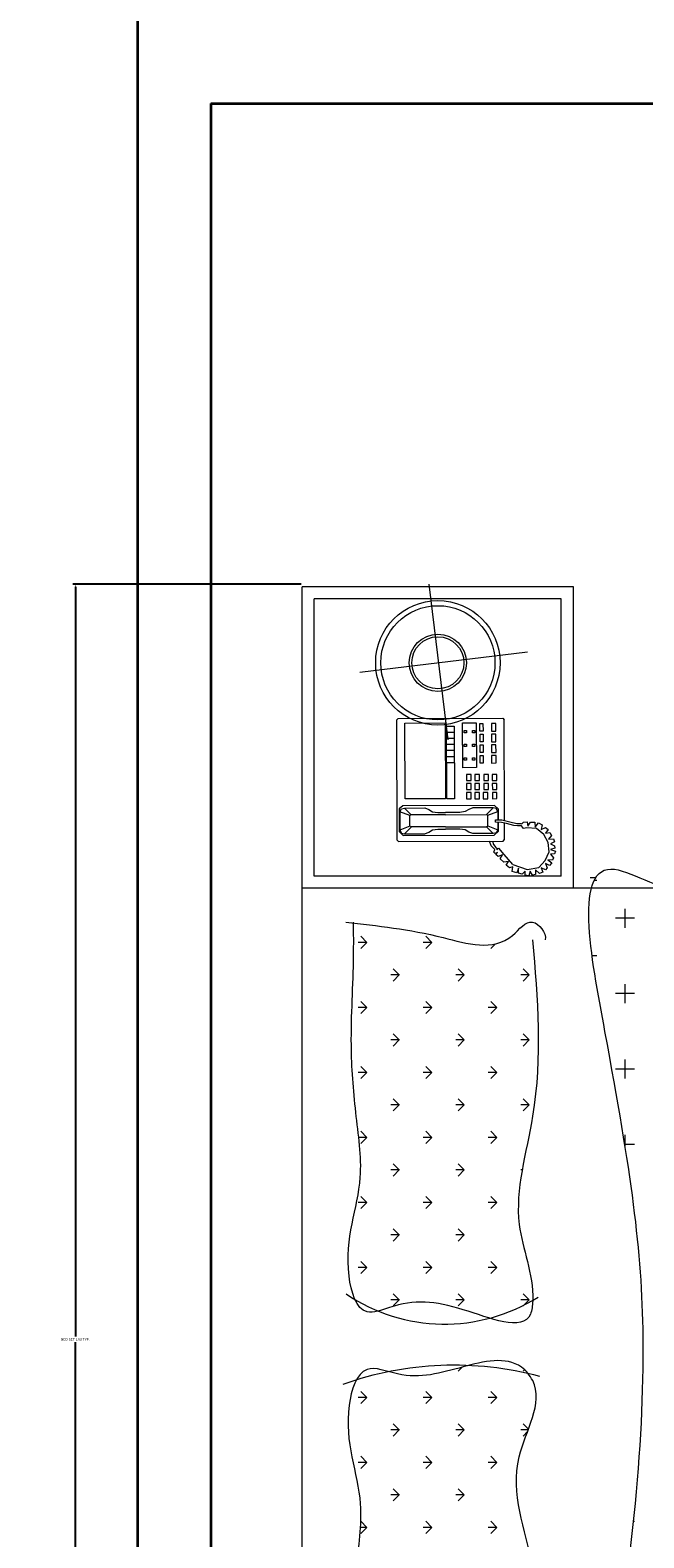
# Model space of a CAD drawing. Units: inches. Extents: x 3731 to 4318, y 1310 to 2388.
# Tile 4 of 57: x 3828 to 3870, y 1452 to 1554. Entities that reach past the tile are written whole.
import ezdxf

# ---------------------------------------------------------------- set-up
doc = ezdxf.new("R2010")
doc.units = ezdxf.units.IN
for name, color, linetype, lineweight in [('A-ANNO-DIMS', 2, 'Continuous', 18), ('A-FURN', 8, 'Continuous', 13), ('A-WALL', 7, 'Continuous', 35)]:
    doc.layers.add(name, color=color, linetype=linetype, lineweight=lineweight)
doc.styles.get("Standard").update_dxf_attribs({"font": 'arial.ttf'})
doc.dimstyles.get("Standard").update_dxf_attribs({"dimtxt": 0.18, "dimasz": 0.18, "dimexe": 0.18, "dimexo": 0.0625, "dimgap": 0.09, "dimtad": 0, "dimtih": 1, "dimtoh": 1, "dimdec": 4, "dimzin": 0, "dimdsep": 46, "dimtxsty": 'Standard', "dimcen": 0.09, "dimadec": 0, "dimazin": 0, "dimtfac": 1, "dimtdec": 4, "dimtofl": 0, "dimtmove": 0, "dimatfit": 3, "dimfxl": 1, "dimtolj": 1, "dimtzin": 0, "dimarcsym": 0})

# ---------------------------------------------------------------- blocks, each defined once
blk = doc.blocks.new('A$C200C7901')
for p, q in [((0.5, 2.3334), (2, 2.3334)), ((2, 2.3334), (2.5, 2.3334)), ((2, 1.6055), (2, 2.3334)), ((2.5, 1.8834), (2.5, 2.3334)), ((0.9943, 2.1721), (0.9842, 2.1822)), ((0.9943, 2.1721), (0.9842, 2.1822)), ((1.3176, 2.1721), (1.3075, 2.1822)), ((1.3176, 2.1721), (1.3075, 2.1822)), ((0.9943, 2.0643), (0.9842, 2.0744)), ((0.9943, 2.0643), (0.9842, 2.0744)), ((1.206, 2.0681), (1.1997, 2.0744)), ((1.206, 2.0681), (1.1997, 2.0744)), ((1.2019, 1.9645), (1.1997, 1.9666)), ((1.2019, 1.9645), (1.1997, 1.9666)), ((2, 1.8834), (2.5, 1.8834)), ((2.0171, 1.8467), (2.0171, 1.8556)), ((2.0171, 1.8467), (2.0171, 1.8556)), ((2.0129, 1.8445), (2.0129, 1.849)), ((2.0129, 1.8445), (2.0129, 1.849))]:
    blk.add_line(p, q)
at = {"linetype": 'ByBlock'}
for p, q in [((2.02, 2.3134), (2.48, 2.3134)), ((2.02, 1.9034), (2.02, 2.3134)), ((2.48, 1.9034), (2.48, 2.3134)), ((0.9404, 2.2259), (0.9303, 2.236)), ((0.9404, 2.2259), (0.9303, 2.236)), ((0.9404, 2.2259), (0.9404, 2.2369)), ((0.9404, 2.2259), (0.9404, 2.2369)), ((0.9404, 2.2259), (0.9505, 2.236)), ((0.9404, 2.2259), (0.9505, 2.236)), ((1.0482, 2.2259), (1.0381, 2.236)), ((1.0482, 2.2259), (1.0381, 2.236)), ((1.0482, 2.2259), (1.0482, 2.2402)), ((1.0482, 2.2259), (1.0482, 2.2402)), ((1.0482, 2.2259), (1.0583, 2.236)), ((1.0482, 2.2259), (1.0583, 2.236)), ((1.1559, 2.2259), (1.1458, 2.236)), ((1.1559, 2.2259), (1.1458, 2.236)), ((1.1559, 2.2259), (1.1559, 2.2402)), ((1.1559, 2.2259), (1.1559, 2.2402)), ((1.1559, 2.2259), (1.166, 2.236)), ((1.1559, 2.2259), (1.166, 2.236)), ((1.3714, 2.2259), (1.3613, 2.236)), ((1.3714, 2.2259), (1.3613, 2.236)), ((1.3714, 2.2259), (1.3714, 2.2402)), ((1.3714, 2.2259), (1.3714, 2.2402)), ((1.3714, 2.2259), (1.3815, 2.236)), ((1.3714, 2.2259), (1.3815, 2.236)), ((1.4792, 2.2259), (1.4691, 2.236)), ((1.4792, 2.2259), (1.4691, 2.236)), ((1.4792, 2.2259), (1.4792, 2.2402)), ((1.4792, 2.2259), (1.4792, 2.2402)), ((1.4792, 2.2259), (1.4893, 2.236)), ((1.4792, 2.2259), (1.4893, 2.236)), ((1.587, 2.2259), (1.5769, 2.236)), ((1.587, 2.2259), (1.5769, 2.236)), ((1.587, 2.2259), (1.587, 2.2393)), ((1.587, 2.2259), (1.587, 2.2393)), ((1.587, 2.2259), (1.5971, 2.236)), ((1.587, 2.2259), (1.5971, 2.236)), ((1.6947, 2.2259), (1.6846, 2.236)), ((1.6947, 2.2259), (1.6846, 2.236)), ((1.6947, 2.2259), (1.6947, 2.2402)), ((1.6947, 2.2259), (1.6947, 2.2402)), ((1.6947, 2.2259), (1.7048, 2.236)), ((1.6947, 2.2259), (1.7048, 2.236)), ((1.8025, 2.2259), (1.7924, 2.236)), ((1.8025, 2.2259), (1.7924, 2.236)), ((1.8025, 2.2259), (1.8025, 2.2402)), ((1.8025, 2.2259), (1.8025, 2.2402)), ((1.8025, 2.2259), (1.8126, 2.236)), ((1.8025, 2.2259), (1.8126, 2.236)), ((1.9103, 2.2259), (1.9002, 2.236)), ((1.9103, 2.2259), (1.9002, 2.236)), ((1.9103, 2.2259), (1.9103, 2.2402)), ((1.9103, 2.2259), (1.9103, 2.2402)), ((1.9103, 2.2259), (1.9204, 2.236)), ((1.9103, 2.2259), (1.9204, 2.236)), ((2.3581, 2.2373), (2.3919, 1.9595)), ((0.9943, 2.172), (0.9943, 2.1863)), ((0.9943, 2.172), (0.9943, 2.1863)), ((0.9943, 2.1721), (1.0044, 2.1822)), ((0.9943, 2.1721), (1.0044, 2.1822)), ((1.102, 2.1721), (1.0919, 2.1822)), ((1.102, 2.1721), (1.0919, 2.1822)), ((1.102, 2.172), (1.102, 2.1863)), ((1.102, 2.172), (1.102, 2.1863)), ((1.102, 2.1721), (1.1121, 2.1822)), ((1.102, 2.1721), (1.1121, 2.1822)), ((1.3176, 2.172), (1.3176, 2.1863)), ((1.3176, 2.172), (1.3176, 2.1863)), ((1.3176, 2.1721), (1.3277, 2.1822)), ((1.3176, 2.1721), (1.3277, 2.1822)), ((1.4253, 2.1721), (1.4152, 2.1822)), ((1.4253, 2.1721), (1.4152, 2.1822)), ((1.4253, 2.172), (1.4253, 2.1863)), ((1.4253, 2.172), (1.4253, 2.1863)), ((1.4253, 2.1721), (1.4354, 2.1822)), ((1.4253, 2.1721), (1.4354, 2.1822)), ((1.5331, 2.1721), (1.523, 2.1822)), ((1.5331, 2.1721), (1.523, 2.1822)), ((1.5331, 2.172), (1.5331, 2.1863)), ((1.5331, 2.172), (1.5331, 2.1863)), ((1.5331, 2.1721), (1.5432, 2.1822)), ((1.5331, 2.1721), (1.5432, 2.1822)), ((1.6409, 2.1721), (1.6308, 2.1822)), ((1.6409, 2.1721), (1.6308, 2.1822)), ((1.6408, 2.172), (1.6408, 2.1863)), ((1.6408, 2.172), (1.6408, 2.1863)), ((1.6409, 2.1721), (1.651, 2.1822)), ((1.6409, 2.1721), (1.651, 2.1822)), ((1.7486, 2.1721), (1.7385, 2.1822)), ((1.7486, 2.1721), (1.7385, 2.1822)), ((1.7486, 2.172), (1.7486, 2.1863)), ((1.7486, 2.172), (1.7486, 2.1863)), ((1.7486, 2.1721), (1.7587, 2.1822)), ((1.7486, 2.1721), (1.7587, 2.1822)), ((1.8564, 2.1721), (1.8463, 2.1822)), ((1.8564, 2.1721), (1.8463, 2.1822)), ((1.8564, 2.172), (1.8564, 2.1863)), ((1.8564, 2.172), (1.8564, 2.1863)), ((1.8564, 2.1721), (1.8665, 2.1822)), ((1.8564, 2.1721), (1.8665, 2.1822)), ((2.0802, 2.176), (2.0777, 2.1734)), ((2.2789, 2.1766), (2.0802, 2.176)), ((2.2789, 2.1766), (2.2814, 2.1741)), ((2.0777, 2.1734), (2.0783, 1.9999)), ((2.0941, 2.1722), (2.0878, 2.1659)), ((2.0878, 2.1659), (2.0883, 2.015)), ((2.0915, 2.1685), (2.0903, 2.1634)), ((2.0903, 2.1634), (2.1017, 2.1521)), ((2.0903, 2.1634), (2.0904, 2.1295)), ((2.0966, 2.171), (2.0915, 2.1685)), ((2.1318, 2.1724), (2.0941, 2.1722)), ((2.1267, 2.1711), (2.0966, 2.171)), ((2.1029, 2.1547), (2.0966, 2.171)), ((2.1017, 2.1521), (2.1029, 2.1547)), ((2.1019, 2.0956), (2.1017, 2.1521)), ((2.1029, 2.1547), (2.1205, 2.1547)), ((2.1205, 2.1547), (2.1267, 2.1711)), ((2.1218, 2.1522), (2.1205, 2.1547)), ((2.1331, 2.1636), (2.1218, 2.1522)), ((2.122, 2.0956), (2.1218, 2.1522)), ((2.1267, 2.1711), (2.1318, 2.1686)), ((2.1368, 2.1661), (2.1318, 2.1724)), ((2.1318, 2.1686), (2.1331, 2.1636)), ((2.1331, 2.1636), (2.1332, 2.1296)), ((2.1373, 2.014), (2.1368, 2.1661)), ((2.1481, 2.1624), (2.2739, 2.1628)), ((2.1484, 2.0957), (2.1481, 2.1624)), ((2.2739, 2.1628), (2.2741, 2.0961)), ((2.2814, 2.1741), (2.282, 2.0006)), ((0.9404, 2.1182), (0.9303, 2.1283)), ((0.9404, 2.1182), (0.9303, 2.1283)), ((0.9404, 2.1182), (0.9404, 2.1325)), ((0.9404, 2.1182), (0.9404, 2.1325)), ((0.9404, 2.1182), (0.9505, 2.1283)), ((0.9404, 2.1182), (0.9505, 2.1283)), ((1.0482, 2.1182), (1.0381, 2.1283)), ((1.0482, 2.1182), (1.0381, 2.1283)), ((1.0482, 2.1182), (1.0482, 2.1325)), ((1.0482, 2.1182), (1.0482, 2.1325)), ((1.0482, 2.1182), (1.0583, 2.1283)), ((1.0482, 2.1182), (1.0583, 2.1283)), ((1.1559, 2.1182), (1.1458, 2.1283)), ((1.1559, 2.1182), (1.1458, 2.1283)), ((1.1559, 2.1182), (1.1559, 2.1325)), ((1.1559, 2.1182), (1.1559, 2.1325)), ((1.1559, 2.1182), (1.166, 2.1283)), ((1.1559, 2.1182), (1.166, 2.1283)), ((1.3714, 2.1182), (1.3613, 2.1283)), ((1.3714, 2.1182), (1.3613, 2.1283)), ((1.3714, 2.1182), (1.3714, 2.1325)), ((1.3714, 2.1182), (1.3714, 2.1325)), ((1.3714, 2.1182), (1.3815, 2.1283)), ((1.3714, 2.1182), (1.3815, 2.1283)), ((1.4792, 2.1182), (1.4691, 2.1283)), ((1.4792, 2.1182), (1.4691, 2.1283)), ((1.4792, 2.1182), (1.4792, 2.1325)), ((1.4792, 2.1182), (1.4792, 2.1325)), ((1.4792, 2.1182), (1.4893, 2.1283)), ((1.4792, 2.1182), (1.4893, 2.1283)), ((1.587, 2.1182), (1.5769, 2.1283)), ((1.587, 2.1182), (1.5769, 2.1283)), ((1.587, 2.1182), (1.587, 2.1325)), ((1.587, 2.1182), (1.587, 2.1325)), ((1.587, 2.1182), (1.5971, 2.1283)), ((1.587, 2.1182), (1.5971, 2.1283)), ((1.6947, 2.1182), (1.6846, 2.1283)), ((1.6947, 2.1182), (1.6846, 2.1283)), ((1.6947, 2.1182), (1.6947, 2.1325)), ((1.6947, 2.1182), (1.6947, 2.1325)), ((1.6947, 2.1182), (1.7048, 2.1283)), ((1.6947, 2.1182), (1.7048, 2.1283)), ((1.8025, 2.1182), (1.7924, 2.1283)), ((1.8025, 2.1182), (1.7924, 2.1283)), ((1.8025, 2.1182), (1.8025, 2.1325)), ((1.8025, 2.1182), (1.8025, 2.1325)), ((1.8025, 2.1182), (1.8126, 2.1283)), ((1.8025, 2.1182), (1.8126, 2.1283)), ((1.9103, 2.1182), (1.9002, 2.1283)), ((1.9103, 2.1182), (1.9002, 2.1283)), ((1.9103, 2.1182), (1.9103, 2.1325)), ((1.9103, 2.1182), (1.9103, 2.1325)), ((1.9103, 2.1182), (1.9204, 2.1283)), ((1.9103, 2.1182), (1.9204, 2.1283)), ((2.0904, 2.1295), (2.093, 2.1232)), ((2.1332, 2.1296), (2.1307, 2.1233)), ((2.093, 2.1232), (2.0968, 2.1169)), ((2.0968, 2.1169), (2.098, 2.1081)), ((2.098, 2.1081), (2.0981, 2.0956)), ((2.1269, 2.117), (2.1257, 2.1082)), ((2.1257, 2.1082), (2.1257, 2.0956)), ((2.1307, 2.1233), (2.1269, 2.117)), ((2.2464, 2.0911), (2.5044, 2.1228)), ((0.9943, 2.0643), (0.9943, 2.0786)), ((0.9943, 2.0643), (0.9943, 2.0786)), ((1.102, 2.0643), (1.102, 2.0786)), ((1.102, 2.0643), (1.102, 2.0786)), ((1.3176, 2.0643), (1.3176, 2.0786)), ((1.3176, 2.0643), (1.3176, 2.0786)), ((1.4253, 2.0643), (1.4253, 2.0786)), ((1.4253, 2.0643), (1.4253, 2.0786)), ((1.5331, 2.0643), (1.5331, 2.0786)), ((1.5331, 2.0643), (1.5331, 2.0786)), ((1.6408, 2.0643), (1.6408, 2.0786)), ((1.6408, 2.0643), (1.6408, 2.0786)), ((1.7486, 2.0643), (1.7486, 2.0786)), ((1.7486, 2.0643), (1.7486, 2.0786)), ((1.8564, 2.0643), (1.8564, 2.0786)), ((1.8564, 2.0643), (1.8564, 2.0786)), ((2.0982, 2.0717), (2.0981, 2.0956)), ((2.1019, 2.0956), (2.1021, 2.0277)), ((2.122, 2.0956), (2.1222, 2.0277)), ((2.1258, 2.0718), (2.1257, 2.0956)), ((2.2741, 2.0961), (2.1484, 2.0957)), ((2.1484, 2.0932), (2.2691, 2.0936)), ((2.1484, 2.0806), (2.1484, 2.0932)), ((2.2691, 2.081), (2.1484, 2.0806)), ((2.2087, 2.0934), (2.2088, 2.0808)), ((2.2188, 2.0934), (2.2188, 2.0809)), ((2.2288, 2.0935), (2.2289, 2.0809)), ((2.2389, 2.0935), (2.239, 2.0809)), ((2.249, 2.0935), (2.249, 2.081)), ((2.259, 2.0936), (2.2591, 2.081)), ((2.2691, 2.0936), (2.2691, 2.081)), ((0.9943, 2.0643), (1.0044, 2.0744)), ((0.9943, 2.0643), (1.0044, 2.0744)), ((1.102, 2.0643), (1.0919, 2.0744)), ((1.102, 2.0643), (1.0919, 2.0744)), ((1.102, 2.0643), (1.1121, 2.0744)), ((1.102, 2.0643), (1.1121, 2.0744)), ((1.3176, 2.0643), (1.3075, 2.0744)), ((1.3176, 2.0643), (1.3075, 2.0744)), ((1.3176, 2.0643), (1.3277, 2.0744)), ((1.3176, 2.0643), (1.3277, 2.0744)), ((1.4253, 2.0643), (1.4152, 2.0744)), ((1.4253, 2.0643), (1.4152, 2.0744)), ((1.4253, 2.0643), (1.4354, 2.0744)), ((1.4253, 2.0643), (1.4354, 2.0744)), ((1.5331, 2.0643), (1.523, 2.0744)), ((1.5331, 2.0643), (1.523, 2.0744)), ((1.5331, 2.0643), (1.5432, 2.0744)), ((1.5331, 2.0643), (1.5432, 2.0744)), ((1.6409, 2.0643), (1.6308, 2.0744)), ((1.6409, 2.0643), (1.6308, 2.0744)), ((1.6409, 2.0643), (1.651, 2.0744)), ((1.6409, 2.0643), (1.651, 2.0744)), ((1.7486, 2.0643), (1.7385, 2.0744)), ((1.7486, 2.0643), (1.7385, 2.0744)), ((1.7486, 2.0643), (1.7587, 2.0744)), ((1.7486, 2.0643), (1.7587, 2.0744)), ((1.8564, 2.0643), (1.8463, 2.0744)), ((1.8564, 2.0643), (1.8463, 2.0744)), ((1.8564, 2.0643), (1.8665, 2.0744)), ((1.8564, 2.0643), (1.8665, 2.0744)), ((2.0907, 2.0503), (2.0932, 2.0566)), ((2.0908, 2.0163), (2.0907, 2.0503)), ((2.0932, 2.0566), (2.0969, 2.0629)), ((2.0969, 2.0629), (2.0982, 2.0717)), ((2.1271, 2.063), (2.1258, 2.0718)), ((2.1309, 2.0567), (2.1271, 2.063)), ((2.1334, 2.0504), (2.1309, 2.0567)), ((2.1336, 2.0165), (2.1334, 2.0504)), ((2.1586, 2.0606), (2.1485, 2.0605)), ((2.1485, 2.0605), (2.1485, 2.053)), ((2.1485, 2.053), (2.1586, 2.053)), ((2.1586, 2.053), (2.1586, 2.0606)), ((2.1636, 2.0606), (2.1636, 2.053)), ((2.1736, 2.0606), (2.1636, 2.0606)), ((2.1636, 2.053), (2.1737, 2.0531)), ((2.1737, 2.0531), (2.1736, 2.0606)), ((2.1887, 2.0607), (2.1787, 2.0606)), ((2.1787, 2.0606), (2.1787, 2.0531)), ((2.1787, 2.0531), (2.1888, 2.0531)), ((2.1888, 2.0531), (2.1887, 2.0607)), ((2.2, 2.067), (2.2742, 2.0672)), ((2.2001, 2.0443), (2.2, 2.067)), ((2.2126, 2.0645), (2.2164, 2.0645)), ((2.2126, 2.0607), (2.2126, 2.0645)), ((2.2164, 2.0607), (2.2126, 2.0607)), ((2.2126, 2.0507), (2.2164, 2.0507)), ((2.2127, 2.0469), (2.2126, 2.0507)), ((2.2164, 2.0645), (2.2164, 2.0607)), ((2.2164, 2.0507), (2.2164, 2.0469)), ((2.2352, 2.0646), (2.239, 2.0646)), ((2.2352, 2.0608), (2.2352, 2.0646)), ((2.239, 2.0608), (2.2352, 2.0608)), ((2.2353, 2.0508), (2.2391, 2.0508)), ((2.2353, 2.047), (2.2353, 2.0508)), ((2.239, 2.0646), (2.239, 2.0608)), ((2.2391, 2.0508), (2.2391, 2.047)), ((2.2579, 2.0609), (2.2579, 2.0647)), ((2.2579, 2.0647), (2.2616, 2.0647)), ((2.2616, 2.0609), (2.2579, 2.0609)), ((2.2579, 2.0508), (2.2617, 2.0508)), ((2.2579, 2.0471), (2.2579, 2.0508)), ((2.2616, 2.0647), (2.2616, 2.0609)), ((2.2617, 2.0508), (2.2617, 2.0471)), ((2.2742, 2.0672), (2.2743, 2.0446)), ((2.0908, 2.0163), (2.1021, 2.0277)), ((2.1034, 2.0252), (2.0971, 2.0088)), ((2.1021, 2.0277), (2.1034, 2.0252)), ((2.1034, 2.0252), (2.121, 2.0252)), ((2.1222, 2.0277), (2.121, 2.0252)), ((2.121, 2.0252), (2.1273, 2.0089)), ((2.1336, 2.0165), (2.1222, 2.0277)), ((2.1485, 2.0467), (2.1486, 2.0391)), ((2.1586, 2.0467), (2.1485, 2.0467)), ((2.1486, 2.0391), (2.1586, 2.0392)), ((2.1586, 2.0329), (2.1486, 2.0329)), ((2.1486, 2.0329), (2.1486, 2.0253)), ((2.1486, 2.0253), (2.1587, 2.0253)), ((2.1586, 2.0392), (2.1586, 2.0467)), ((2.1587, 2.0253), (2.1586, 2.0329)), ((2.1737, 2.0468), (2.1636, 2.0467)), ((2.1636, 2.0467), (2.1637, 2.0392)), ((2.1637, 2.0392), (2.1737, 2.0392)), ((2.1637, 2.0317), (2.1637, 2.0241)), ((2.1737, 2.0317), (2.1637, 2.0317)), ((2.1737, 2.0392), (2.1737, 2.0468)), ((2.1738, 2.0241), (2.1737, 2.0317)), ((2.1787, 2.0468), (2.1787, 2.0392)), ((2.1888, 2.0468), (2.1787, 2.0468)), ((2.1787, 2.0392), (2.1888, 2.0393)), ((2.1788, 2.0317), (2.1788, 2.0242)), ((2.1888, 2.0317), (2.1788, 2.0317)), ((2.1888, 2.0393), (2.1888, 2.0468)), ((2.1889, 2.0242), (2.1888, 2.0317)), ((2.2743, 2.0446), (2.2001, 2.0443)), ((2.2077, 2.0331), (2.2077, 2.0381)), ((2.2077, 2.0381), (2.2202, 2.0381)), ((2.2203, 2.0331), (2.2077, 2.0331)), ((2.2164, 2.0469), (2.2127, 2.0469)), ((2.2202, 2.0381), (2.2203, 2.0331)), ((2.2253, 2.0381), (2.2378, 2.0382)), ((2.2253, 2.0331), (2.2253, 2.0381)), ((2.2379, 2.0332), (2.2253, 2.0331)), ((2.2391, 2.047), (2.2353, 2.047)), ((2.2378, 2.0382), (2.2379, 2.0332)), ((2.2429, 2.0332), (2.2429, 2.0382)), ((2.2429, 2.0382), (2.2554, 2.0382)), ((2.2555, 2.0332), (2.2429, 2.0332)), ((2.2554, 2.0382), (2.2555, 2.0332)), ((2.2617, 2.0471), (2.2579, 2.0471)), ((2.2605, 2.0332), (2.2605, 2.0383)), ((2.2605, 2.0383), (2.273, 2.0383)), ((2.2731, 2.0333), (2.2605, 2.0332)), ((2.273, 2.0383), (2.2731, 2.0333)), ((0.9404, 2.0104), (0.9303, 2.0205)), ((0.9404, 2.0104), (0.9303, 2.0205)), ((0.9404, 2.0104), (0.9404, 2.0247)), ((0.9404, 2.0104), (0.9404, 2.0247)), ((0.9404, 2.0104), (0.9505, 2.0205)), ((0.9404, 2.0104), (0.9505, 2.0205)), ((1.0482, 2.0104), (1.0381, 2.0205)), ((1.0482, 2.0104), (1.0381, 2.0205)), ((1.0482, 2.0104), (1.0482, 2.0247)), ((1.0482, 2.0104), (1.0482, 2.0247)), ((1.0482, 2.0104), (1.0583, 2.0205)), ((1.0482, 2.0104), (1.0583, 2.0205)), ((1.1559, 2.0104), (1.1458, 2.0205)), ((1.1559, 2.0104), (1.1458, 2.0205)), ((1.1559, 2.0104), (1.1559, 2.0247)), ((1.1559, 2.0104), (1.1559, 2.0247)), ((1.1559, 2.0104), (1.166, 2.0205)), ((1.1559, 2.0104), (1.166, 2.0205)), ((1.3714, 2.0104), (1.3613, 2.0205)), ((1.3714, 2.0104), (1.3613, 2.0205)), ((1.3714, 2.0104), (1.3714, 2.0247)), ((1.3714, 2.0104), (1.3714, 2.0247)), ((1.3714, 2.0104), (1.3815, 2.0205)), ((1.3714, 2.0104), (1.3815, 2.0205)), ((1.4792, 2.0104), (1.4691, 2.0205)), ((1.4792, 2.0104), (1.4691, 2.0205)), ((1.4792, 2.0104), (1.4792, 2.0247)), ((1.4792, 2.0104), (1.4792, 2.0247)), ((1.4792, 2.0104), (1.4893, 2.0205)), ((1.4792, 2.0104), (1.4893, 2.0205)), ((1.587, 2.0104), (1.5769, 2.0205)), ((1.587, 2.0104), (1.5769, 2.0205)), ((1.587, 2.0104), (1.587, 2.0247)), ((1.587, 2.0104), (1.587, 2.0247)), ((1.587, 2.0104), (1.5971, 2.0205)), ((1.587, 2.0104), (1.5971, 2.0205)), ((1.6947, 2.0104), (1.6846, 2.0205)), ((1.6947, 2.0104), (1.6846, 2.0205)), ((1.6947, 2.0104), (1.6947, 2.0247)), ((1.6947, 2.0104), (1.6947, 2.0247)), ((1.6947, 2.0104), (1.7048, 2.0205)), ((1.6947, 2.0104), (1.7048, 2.0205)), ((1.8025, 2.0104), (1.7924, 2.0205)), ((1.8025, 2.0104), (1.7924, 2.0205)), ((1.8025, 2.0104), (1.8025, 2.0247)), ((1.8025, 2.0104), (1.8025, 2.0247)), ((1.8025, 2.0104), (1.8126, 2.0205)), ((1.8025, 2.0104), (1.8126, 2.0205)), ((1.9068, 2.0139), (1.9002, 2.0205)), ((1.9068, 2.0139), (1.9002, 2.0205)), ((2.0431, 1.999), (2.0488, 2.0046)), ((2.0488, 2.0046), (2.0557, 2.0011)), ((2.053, 2.0084), (2.0563, 2.0119)), ((2.0557, 2.0011), (2.053, 2.0084)), ((2.0663, 2.0077), (2.0561, 1.9986)), ((2.0563, 2.0119), (2.0594, 2.0095)), ((2.0576, 2.0133), (2.0598, 2.0155)), ((2.0594, 2.0095), (2.0576, 2.0133)), ((2.0598, 2.0155), (2.0645, 2.0137)), ((2.0663, 2.0102), (2.0636, 2.0104)), ((2.0636, 2.0104), (2.0663, 2.0077)), ((2.0645, 2.0137), (2.0671, 2.0162)), ((2.0676, 2.012), (2.0663, 2.0102)), ((2.0671, 2.0162), (2.0707, 2.0197)), ((2.0727, 2.016), (2.0676, 2.012)), ((2.0707, 2.0197), (2.0782, 2.0226)), ((2.0782, 2.0175), (2.0727, 2.016)), ((2.0783, 1.9999), (2.0808, 1.9974)), ((2.0883, 2.015), (2.0946, 2.0075)), ((2.0921, 2.0113), (2.0908, 2.0163)), ((2.0971, 2.0088), (2.0921, 2.0113)), ((2.0946, 2.0075), (2.1093, 2.0076)), ((2.1094, 2.0088), (2.0971, 2.0088)), ((2.1072, 1.9944), (2.109, 2.0025)), ((2.109, 2.0025), (2.1097, 2.0126)), ((2.1097, 2.0126), (2.1135, 2.0126)), ((2.1133, 2.0018), (2.1103, 1.989)), ((2.1135, 2.0126), (2.1133, 2.0018)), ((2.1273, 2.0089), (2.1134, 2.0088)), ((2.1134, 2.0076), (2.1311, 2.0077)), ((2.1273, 2.0089), (2.1323, 2.0114)), ((2.1311, 2.0077), (2.1373, 2.014)), ((2.1323, 2.0114), (2.1336, 2.0165)), ((2.1587, 2.0178), (2.1486, 2.0178)), ((2.1486, 2.0178), (2.1487, 2.0102)), ((2.1487, 2.0102), (2.1587, 2.0103)), ((2.1587, 2.0103), (2.1587, 2.0178)), ((2.1637, 2.0241), (2.1738, 2.0241)), ((2.1738, 2.0179), (2.1637, 2.0178)), ((2.1637, 2.0178), (2.1638, 2.0103)), ((2.1638, 2.0103), (2.1738, 2.0103)), ((2.1738, 2.0103), (2.1738, 2.0179)), ((2.1788, 2.0242), (2.1889, 2.0242)), ((2.1788, 2.0179), (2.1788, 2.0103)), ((2.1889, 2.0179), (2.1788, 2.0179)), ((2.1788, 2.0103), (2.1889, 2.0104)), ((2.1889, 2.0104), (2.1889, 2.0179)), ((2.2203, 2.0193), (2.2077, 2.0192)), ((2.2077, 2.0192), (2.2078, 2.0117)), ((2.2078, 2.0117), (2.2203, 2.0117)), ((2.2203, 2.0117), (2.2203, 2.0193)), ((2.2379, 2.0193), (2.2253, 2.0193)), ((2.2253, 2.0193), (2.2254, 2.0117)), ((2.2254, 2.0117), (2.2379, 2.0118)), ((2.2379, 2.0118), (2.2379, 2.0193)), ((2.2555, 2.0194), (2.2429, 2.0193)), ((2.2429, 2.0193), (2.243, 2.0118)), ((2.243, 2.0118), (2.2555, 2.0118)), ((2.2555, 2.0118), (2.2555, 2.0194)), ((2.2605, 2.0194), (2.2606, 2.0119)), ((2.2731, 2.0194), (2.2605, 2.0194)), ((2.2606, 2.0119), (2.2731, 2.0119)), ((2.2731, 2.0119), (2.2731, 2.0194)), ((2.282, 2.0006), (2.2795, 1.9981)), ((2.0259, 1.977), (2.0281, 1.9847)), ((2.0333, 1.9743), (2.0259, 1.977)), ((2.0281, 1.9847), (2.0358, 1.9839)), ((2.0393, 1.984), (2.031, 1.96)), ((2.0338, 1.9895), (2.0386, 1.9946)), ((2.0358, 1.9839), (2.0338, 1.9895)), ((2.0386, 1.9946), (2.0444, 1.9911)), ((2.0561, 1.9986), (2.0396, 1.9844)), ((2.0444, 1.9911), (2.0431, 1.999)), ((2.0808, 1.9974), (2.1079, 1.9975)), ((2.1035, 1.9763), (2.1042, 1.9824)), ((2.1038, 1.9697), (2.1035, 1.9763)), ((2.1042, 1.9824), (2.1072, 1.9944)), ((2.1103, 1.989), (2.1073, 1.9771)), ((2.1073, 1.9771), (2.1076, 1.9704)), ((2.1123, 1.9975), (2.2795, 1.9981)), ((1.0993, 1.9593), (1.0919, 1.9666)), ((1.0993, 1.9593), (1.0919, 1.9666)), ((1.102, 1.9583), (1.102, 1.9708)), ((1.102, 1.9583), (1.102, 1.9708)), ((1.1033, 1.9578), (1.1121, 1.9666)), ((1.1033, 1.9578), (1.1121, 1.9666)), ((1.3176, 1.9565), (1.3075, 1.9666)), ((1.3176, 1.9565), (1.3075, 1.9666)), ((1.3176, 1.9565), (1.3176, 1.9708)), ((1.3176, 1.9565), (1.3176, 1.9708)), ((1.3176, 1.9565), (1.3277, 1.9666)), ((1.3176, 1.9565), (1.3277, 1.9666)), ((1.4253, 1.9703), (1.4253, 1.9708)), ((1.4253, 1.9703), (1.4253, 1.9708)), ((1.5331, 1.9683), (1.5331, 1.9708)), ((1.5331, 1.9683), (1.5331, 1.9708)), ((1.543, 1.9665), (1.5432, 1.9666)), ((1.543, 1.9665), (1.5432, 1.9666)), ((1.6409, 1.9565), (1.6308, 1.9666)), ((1.6409, 1.9565), (1.6308, 1.9666)), ((1.6408, 1.9565), (1.6408, 1.9708)), ((1.6408, 1.9565), (1.6408, 1.9708)), ((1.6409, 1.9565), (1.651, 1.9666)), ((1.6409, 1.9565), (1.651, 1.9666)), ((1.7486, 1.9565), (1.7385, 1.9666)), ((1.7486, 1.9565), (1.7385, 1.9666)), ((1.7486, 1.9565), (1.7486, 1.9708)), ((1.7486, 1.9565), (1.7486, 1.9708)), ((1.7486, 1.9565), (1.7587, 1.9666)), ((1.7486, 1.9565), (1.7587, 1.9666)), ((1.8564, 1.9565), (1.8463, 1.9666)), ((1.8564, 1.9565), (1.8463, 1.9666)), ((1.8564, 1.9565), (1.8564, 1.9708)), ((1.8564, 1.9565), (1.8564, 1.9708)), ((1.8564, 1.9565), (1.8665, 1.9666)), ((1.8564, 1.9565), (1.8665, 1.9666)), ((2.0206, 1.9572), (2.0218, 1.9635)), ((2.0285, 1.9549), (2.0206, 1.9572)), ((2.0218, 1.9635), (2.0287, 1.9636)), ((2.0219, 1.9511), (2.0285, 1.9549)), ((2.0229, 1.946), (2.0219, 1.9511)), ((2.0234, 1.9686), (2.0251, 1.9745)), ((2.0287, 1.9636), (2.0234, 1.9686)), ((2.0251, 1.9745), (2.0333, 1.9743)), ((2.031, 1.96), (2.0346, 1.9409)), ((2.099, 1.9444), (2.1002, 1.9605)), ((2.0992, 1.9663), (2.1038, 1.9697)), ((2.1002, 1.9605), (2.0992, 1.9663)), ((2.1101, 1.96), (2.1028, 1.9587)), ((2.1028, 1.9587), (2.1099, 1.9544)), ((2.1076, 1.9704), (2.1068, 1.9689)), ((2.1068, 1.9689), (2.1096, 1.9661)), ((2.1099, 1.9544), (2.1094, 1.9475)), ((2.1096, 1.9661), (2.1101, 1.96)), ((2.0308, 1.9462), (2.0229, 1.946)), ((2.0247, 1.9394), (2.0308, 1.9462)), ((2.0268, 1.9343), (2.0247, 1.9394)), ((2.0341, 1.9366), (2.0268, 1.9343)), ((2.0306, 1.9297), (2.0341, 1.9366)), ((2.0339, 1.9267), (2.0306, 1.9297)), ((2.041, 1.9297), (2.0339, 1.9267)), ((2.0346, 1.9409), (2.0459, 1.93)), ((2.038, 1.9228), (2.041, 1.9297)), ((2.0474, 1.9259), (2.0421, 1.9193)), ((2.0459, 1.93), (2.0607, 1.9237)), ((2.0467, 1.9183), (2.0474, 1.9259)), ((2.0607, 1.9237), (2.0759, 1.925)), ((2.0759, 1.925), (2.0894, 1.9322)), ((2.0894, 1.9322), (2.099, 1.9444)), ((2.0973, 1.9251), (2.0914, 1.9294)), ((2.0914, 1.9294), (2.0925, 1.9225)), ((2.1011, 1.9297), (2.0973, 1.9251)), ((2.1051, 1.9353), (2.0975, 1.9368)), ((2.0975, 1.9368), (2.1011, 1.9297)), ((2.1094, 1.9475), (2.1013, 1.9467)), ((2.1013, 1.9467), (2.1084, 1.9412)), ((2.1084, 1.9412), (2.1051, 1.9353)), ((2.02, 1.9034), (2.48, 1.9034)), ((2.0421, 1.9193), (2.038, 1.9228)), ((2.0508, 1.9163), (2.0467, 1.9183)), ((2.0566, 1.9214), (2.0508, 1.9163)), ((2.0569, 1.9145), (2.0566, 1.9214)), ((2.0617, 1.9133), (2.0569, 1.9145)), ((2.0645, 1.9214), (2.0617, 1.9133)), ((2.0663, 1.914), (2.0645, 1.9214)), ((2.0706, 1.9146), (2.0663, 1.914)), ((2.0736, 1.9214), (2.0706, 1.9146)), ((2.077, 1.9146), (2.0736, 1.9214)), ((2.0823, 1.9161), (2.077, 1.9146)), ((2.0876, 1.9195), (2.0815, 1.9245)), ((2.0815, 1.9245), (2.0823, 1.9161)), ((2.0925, 1.9225), (2.0876, 1.9195)), ((1.8879, 1.8445), (1.8879, 1.8523)), ((1.8879, 1.8445), (1.8879, 1.8523)), ((1.7004, 1.782), (1.7004, 1.8133)), ((1.7004, 1.782), (1.7004, 1.8133)), ((1.8254, 1.782), (1.8254, 1.8133)), ((1.8254, 1.782), (1.8254, 1.8133)), ((1.9504, 1.782), (1.9504, 1.8133)), ((1.9504, 1.782), (1.9504, 1.8133)), ((0.9504, 1.782), (0.9504, 1.7836)), ((0.9504, 1.782), (0.9504, 1.7836)), ((1.573, 1.7977), (1.591, 1.7977)), ((1.573, 1.7977), (1.591, 1.7977)), ((1.5754, 1.782), (1.5754, 1.7981)), ((1.5754, 1.782), (1.5754, 1.7981)), ((1.6847, 1.7977), (1.716, 1.7977)), ((1.6847, 1.7977), (1.716, 1.7977)), ((1.8097, 1.7977), (1.841, 1.7977)), ((1.8097, 1.7977), (1.841, 1.7977)), ((1.9347, 1.7977), (1.966, 1.7977)), ((1.9347, 1.7977), (1.966, 1.7977))]:
    blk.add_line(p, q, dxfattribs=at)
for radius in [0.1032, 0.0947, 0.0475, 0.0432]:
    blk.add_circle((2.3739, 2.1081), radius, dxfattribs=at)
for centre, radius, start, end in [((0.658, 2.0811), 0.5513, 345.0722, 19.5492), ((1.5685, 2.097), 0.291, 145.8603, 212.2445)]:
    blk.add_arc(centre, radius, start, end)
for points, knots in [([(0.5854, 1.951), (0.6835, 1.9407), (0.8425, 1.9242), (1.0374, 2.0054), (1.1564, 1.9255), (1.2274, 1.9841), (1.2052, 2.0751), (1.1815, 2.152), (1.2176, 2.2368), (1.0992, 2.2731), (1.0008, 2.2255), (0.8698, 2.246), (0.7481, 2.2548), (0.6426, 2.2473), (0.5746, 2.2478), (0.5562, 2.2479)], [0, 0, 0, 0, 292.165466, 473.33038, 601.631673, 630.723769, 727.138505, 836.819956, 887.958136, 954.42438, 1118.989809, 1227.016542, 1338.750986, 1487.447361, 1542.751028, 1542.751028, 1542.751028, 1542.751028]), ([(1.9146, 1.951), (1.8174, 1.9428), (1.6601, 1.9297), (1.4574, 1.9942), (1.3549, 1.9462), (1.2593, 1.9563), (1.314, 2.0834), (1.3193, 2.1569), (1.2853, 2.2393), (1.4031, 2.2724), (1.4987, 2.2256), (1.6304, 2.2459), (1.7519, 2.2548), (1.8574, 2.2473), (1.9254, 2.2478), (1.9438, 2.2479)], [0, 0, 0, 0, 292.165466, 473.33038, 601.631673, 624.236147, 735.870502, 858.452188, 896.317728, 962.783971, 1127.3494, 1235.376134, 1347.110578, 1495.806953, 1551.11062, 1551.11062, 1551.11062, 1551.11062]), ([(1.9438, 2.2608), (1.9381, 2.2086), (1.9282, 2.1195), (1.8897, 2.0022), (1.9591, 1.9538), (1.9264, 1.9278), (1.9146, 1.93)], [0, 0, 0, 0, 163.411291, 278.570782, 318.445997, 354.484131, 354.484131, 354.484131, 354.484131]), ([(0.4485, 1.7835), (0.4321, 1.7496), (0.4062, 1.6964), (0.49, 1.6713), (0.4719, 1.5969), (0.4123, 1.592), (0.4233, 1.5337), (0.4954, 1.5086), (0.4012, 1.4738), (0.3253, 1.4306), (0.4113, 1.3764), (0.3688, 1.3065), (0.5579, 1.2663), (0.741, 1.4533), (1.1127, 1.1109), (1.4811, 1.2478), (1.7885, 1.3492), (2.0357, 1.1637), (2.0748, 1.2974), (2.0876, 1.349), (2.0192, 1.3805), (2.0564, 1.4298), (2.0588, 1.4846), (1.9759, 1.5349), (2.1004, 1.5845), (2.0397, 1.6519), (1.971, 1.7053), (2.1104, 1.8981), (1.5946, 1.7967), (1.2448, 1.7472), (0.8129, 1.7935), (0.4953, 1.8548), (0.4582, 1.7983), (0.4485, 1.7835)], [0, 0, 0, 0, 88.420092, 139.08588, 204.302936, 239.695496, 287.801042, 327.365471, 412.960499, 463.626286, 552.059846, 584.668336, 662.614915, 940.993281, 1309.926334, 1844.022653, 1996.276242, 2316.43048, 2341.441004, 2404.707416, 2449.463774, 2514.680778, 2538.40571, 2613.031547, 2697.13096, 2760.903931, 2822.692699, 2945.47, 3215.060018, 3725.584917, 4361.974444, 4504.671998, 4555.32777, 4555.32777, 4555.32777, 4555.32777])]:
    blk.add_open_spline(points, degree=3, knots=knots)
blk = doc.blocks.new('*D16')
at = {"layer": 'A-ANNO-DIMS', "color": 0, "lineweight": -2, "transparency": 16777216}
for p, q in [((3846.36, 1516.63), (3830.8, 1516.63)), ((3830.98, 1516.45), (3830.98, 1465.34)), ((3830.98, 1413.86), (3830.98, 1464.97)), ((3846.36, 1413.68), (3830.8, 1413.68))]:
    blk.add_line(p, q, dxfattribs=at)
at = {"layer": 'A-ANNO-DIMS', "color": 0, "transparency": 16777216}
for points in [[(3830.95, 1516.45), (3831.01, 1516.45), (3830.98, 1516.63)], [(3830.95, 1413.86), (3831.01, 1413.86), (3830.98, 1413.68)]]:
    blk.add_solid(points, dxfattribs=at)
at = {"layer": 'Defpoints', "color": 0, "transparency": 16777216}
for p in [(3830.98, 1516.63), (3846.43, 1516.63), (3846.43, 1413.68)]:
    blk.add_point(p, dxfattribs=at)
at = {"layer": 'A-ANNO-DIMS', "color": 0, "transparency": 16777216, "insert": (3830.98, 1465.15), "char_height": 0.18, "attachment_point": 5}
blk.add_mtext('\\A1;BED SET 103 TYP.', dxfattribs=at)
blk = doc.blocks.new('*D32')
at = {"layer": 'A-ANNO-DIMS', "color": 0, "lineweight": -2, "transparency": 16777216}
for p, q in [((4269.21, 1592.32), (4269.21, 1310.25)), ((3835.21, 1359.32), (3835.21, 1310.25)), ((3835.39, 1310.43), (4051.92, 1310.43)), ((4269.03, 1310.43), (4052.5, 1310.43))]:
    blk.add_line(p, q, dxfattribs=at)
at = {"layer": 'A-ANNO-DIMS', "color": 0, "transparency": 16777216}
for points in [[(3835.39, 1310.46), (3835.39, 1310.4), (3835.21, 1310.43)], [(4269.03, 1310.46), (4269.03, 1310.4), (4269.21, 1310.43)]]:
    blk.add_solid(points, dxfattribs=at)
at = {"layer": 'Defpoints', "color": 0, "transparency": 16777216}
for p in [(4269.21, 1592.38), (3835.21, 1359.38), (4269.21, 1310.43)]:
    blk.add_point(p, dxfattribs=at)
at = {"layer": 'A-ANNO-DIMS', "color": 0, "transparency": 16777216, "insert": (4052.21, 1310.43), "char_height": 0.18, "attachment_point": 5}
blk.add_mtext('\\A1;434', dxfattribs=at)
blk = doc.blocks.new('*D33')
at = {"layer": 'A-ANNO-DIMS', "color": 0, "lineweight": -2, "transparency": 16777216}
for p, q in [((3835.15, 2338.38), (3731.41, 2338.38)), ((3731.59, 2338.2), (3731.59, 1849.06)), ((3731.59, 1359.56), (3731.59, 1848.7)), ((3835.15, 1359.38), (3731.41, 1359.38))]:
    blk.add_line(p, q, dxfattribs=at)
at = {"layer": 'A-ANNO-DIMS', "color": 0, "transparency": 16777216}
for points in [[(3731.56, 2338.2), (3731.62, 2338.2), (3731.59, 2338.38)], [(3731.56, 1359.56), (3731.62, 1359.56), (3731.59, 1359.38)]]:
    blk.add_solid(points, dxfattribs=at)
at = {"layer": 'Defpoints', "color": 0, "transparency": 16777216}
for p in [(3731.59, 2338.38), (3835.21, 2338.38), (3835.21, 1359.38)]:
    blk.add_point(p, dxfattribs=at)
at = {"layer": 'A-ANNO-DIMS', "color": 0, "transparency": 16777216, "insert": (3731.59, 1848.88), "char_height": 0.18, "attachment_point": 5}
blk.add_mtext('\\A1;979', dxfattribs=at)

msp = doc.modelspace()

# ---------------------------------------------------------------- linework, layer by layer
at = {"layer": 'A-WALL'}
for p, q in [((3835.21, 2338.38), (3835.21, 1359.38)), ((3840.21, 1549.38), (3906.21, 1549.38)), ((3840.21, 1549.38), (3840.21, 1393.38))]:
    msp.add_line(p, q, dxfattribs=at)

# ---------------------------------------------------------------- block references
at = {"layer": 'A-FURN', "xscale": 41.1071563136412, "yscale": 41.1071563136412, "zscale": 41.1071563136412, "rotation": 90}
msp.add_blockref('A$C200C7901', (3942.35, 1413.68), dxfattribs=at)

# ---------------------------------------------------------------- dimensions: what is measured, and where the dimension line sits
at = {"layer": 'A-ANNO-DIMS'}
dim = msp.add_linear_dim(base=(3731.59, 2338.38), p1=(3835.21, 1359.38), p2=(3835.21, 2338.38), angle=90, dimstyle='Standard', override={"dimdec": 0, "dimlfac": 1, "dimrnd": 0, "dimzin": 0, "dimdsep": 46, "dimlunit": 2}, dxfattribs=at)
dim.commit()
dim.dimension.update_dxf_attribs({"geometry": '*D33', "text_midpoint": (3731.59, 1848.88)})
dim = msp.add_linear_dim(base=(4269.21, 1310.43), p1=(3835.21, 1359.38), p2=(4269.21, 1592.38), dimstyle='Standard', override={"dimdec": 0, "dimlfac": 1, "dimrnd": 0, "dimzin": 0, "dimdsep": 46, "dimlunit": 2}, dxfattribs=at)
dim.commit()
dim.dimension.update_dxf_attribs({"geometry": '*D32', "text_midpoint": (4052.21, 1310.43)})
dim = msp.add_linear_dim(base=(3830.98, 1516.63), p1=(3846.43, 1413.68), p2=(3846.43, 1516.63), angle=90, text='BED SET <> TYP.', dimstyle='Standard', override={"dimdec": 0, "dimlfac": 1, "dimrnd": 0, "dimzin": 0, "dimdsep": 46, "dimlunit": 2}, dxfattribs=at)
dim.commit()
dim.dimension.update_dxf_attribs({"geometry": '*D16', "text_midpoint": (3830.98, 1465.15)})

doc.saveas('drawing.dxf')
